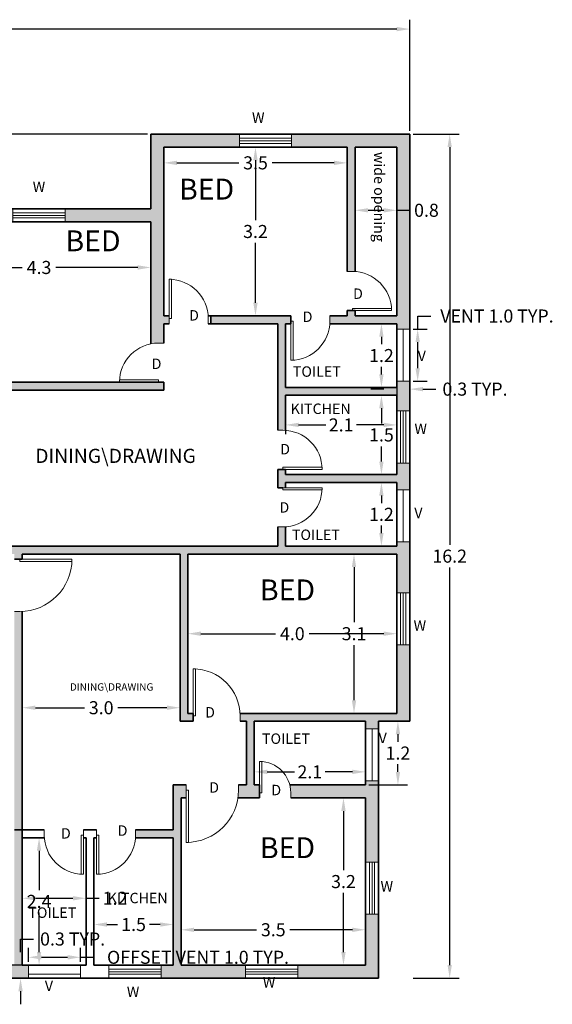
# Model space of a CAD drawing. Units: metres. Extents: x 6.2 to 29.4, y -2.1 to 16.8.
# Tile 3 of 3: x 19.2 to 29.4, y -2.1 to 16.8. Entities that reach past the tile are written whole.
import ezdxf

# ---------------------------------------------------------------- set-up
doc = ezdxf.new("R2010")
doc.units = ezdxf.units.M
doc.header["$MEASUREMENT"] = 0
doc.layers.get('0').update_dxf_attribs({"color": 2})
doc.layers.get('Defpoints').update_dxf_attribs({"color": 3})
for name, color, linetype, lineweight in [('A-ANNO-DIMS', 6, 'Continuous', 13), ('A-ANNO-TEXT', 7, 'Continuous', 18), ('A-AREA-IDEN', 3, 'Continuous', 18), ('A-DOOR', 3, 'Continuous', 18), ('A-GLAZ', 4, 'Continuous', 18), ('A-WALL', 7, 'Continuous', 35), ('A-WALL-PATT', 252, 'Continuous', 13)]:
    doc.layers.add(name, color=color, linetype=linetype, lineweight=lineweight)
doc.styles.get("Standard").update_dxf_attribs({"font": 'arial.ttf'})
doc.dimstyles.get("Standard").update_dxf_attribs({"dimtxt": 0.25, "dimasz": 0.25, "dimexe": 0.18, "dimexo": 0.0625, "dimgap": 0.09, "dimtad": 0, "dimtih": 1, "dimtoh": 1, "dimdec": 1, "dimzin": 0, "dimdsep": 46, "dimtxsty": 'Standard', "dimcen": 0.09, "dimadec": 0, "dimazin": 0, "dimtfac": 1, "dimtdec": 1, "dimtofl": 0, "dimtmove": 0, "dimatfit": 3, "dimfxl": 1, "dimtolj": 1, "dimtzin": 0, "dimarcsym": 0})

# ---------------------------------------------------------------- blocks, each defined once
blk = doc.blocks.new('*U11')
for p, q in [((-750, 0), (-750, 100)), ((0, 0), (0, 100))]:
    blk.add_line(p, q)
blk.add_lwpolyline([(0, 0), (0, -750), (-43.75, -750), (-43.75, 0)], close=True)
blk.add_arc((0, 0), 750, 180, 270)
blk = doc.blocks.new('*D12')
at = {"layer": 'A-ANNO-DIMS', "color": 0, "lineweight": -2, "transparency": 16777216}
for p, q in [((19.462, 1.113), (19.345, 1.113)), ((19.525, 0.863), (19.525, 0.109)), ((19.525, -1.077), (19.525, -0.322)), ((19.462, -1.327), (19.345, -1.327))]:
    blk.add_line(p, q, dxfattribs=at)
at = {"layer": 'A-ANNO-DIMS', "color": 0, "transparency": 16777216}
for points in [[(19.483, 0.863), (19.566, 0.863), (19.525, 1.113)], [(19.483, -1.077), (19.566, -1.077), (19.525, -1.327)]]:
    blk.add_solid(points, dxfattribs=at)
at = {"layer": 'Defpoints', "color": 0, "transparency": 16777216}
for p in [(19.525, 1.113), (19.525, -1.327), (19.525, -1.327)]:
    blk.add_point(p, dxfattribs=at)
at = {"layer": 'A-ANNO-DIMS', "color": 0, "transparency": 16777216, "insert": (19.525, -0.107), "char_height": 0.25, "attachment_point": 5}
blk.add_mtext('\\A1;2.4', dxfattribs=at)
blk = doc.blocks.new('*D13')
at = {"layer": 'A-ANNO-DIMS', "color": 0, "lineweight": -2, "transparency": 16777216}
for p, q in [((19.204, -0.087), (19.204, 0.133)), ((20.424, -1.149), (20.424, 0.133)), ((19.454, -0.047), (20.174, -0.047)), ((20.424, -0.047), (20.674, -0.047))]:
    blk.add_line(p, q, dxfattribs=at)
at = {"layer": 'A-ANNO-DIMS', "color": 0, "transparency": 16777216}
for points in [[(19.454, -0.005), (19.454, -0.088), (19.204, -0.047)], [(20.174, -0.005), (20.174, -0.088), (20.424, -0.047)]]:
    blk.add_solid(points, dxfattribs=at)
at = {"layer": 'Defpoints', "color": 0, "transparency": 16777216}
for p in [(19.204, -0.149), (20.424, -0.047), (20.424, -1.211)]:
    blk.add_point(p, dxfattribs=at)
at = {"layer": 'A-ANNO-DIMS', "color": 0, "transparency": 16777216, "insert": (20.979, -0.047), "char_height": 0.25, "attachment_point": 5}
blk.add_mtext('\\A1;1.2', dxfattribs=at)
blk = doc.blocks.new('*D14')
at = {"layer": 'A-ANNO-DIMS', "color": 0, "lineweight": -2, "transparency": 16777216}
for p, q in [((20.574, -0.487), (20.574, -0.369)), ((22.094, -0.487), (22.094, -0.369)), ((20.824, -0.549), (21.027, -0.549)), ((21.844, -0.549), (21.641, -0.549))]:
    blk.add_line(p, q, dxfattribs=at)
at = {"layer": 'A-ANNO-DIMS', "color": 0, "transparency": 16777216}
for points in [[(20.824, -0.508), (20.824, -0.591), (20.574, -0.549)], [(21.844, -0.508), (21.844, -0.591), (22.094, -0.549)]]:
    blk.add_solid(points, dxfattribs=at)
at = {"layer": 'Defpoints', "color": 0, "transparency": 16777216}
for p in [(20.574, -0.549), (22.094, -0.549), (22.094, -0.549)]:
    blk.add_point(p, dxfattribs=at)
at = {"layer": 'A-ANNO-DIMS', "color": 0, "transparency": 16777216, "insert": (21.334, -0.549), "char_height": 0.25, "attachment_point": 5}
blk.add_mtext('\\A1;1.5', dxfattribs=at)
blk = doc.blocks.new('*U15')
for p, q in [((0, 0), (0, 100)), ((1000, 0), (1000, 100))]:
    blk.add_line(p, q)
blk.add_lwpolyline([(0, 0), (0, -1000), (43.75, -1000), (43.75, 0)], close=True)
blk.add_arc((0, 0), 1000, 270, 0)
blk = doc.blocks.new('*D16')
at = {"layer": 'A-ANNO-DIMS', "color": 0, "lineweight": -2, "transparency": 16777216}
for p, q in [((22.244, -1.264), (22.244, -0.47)), ((25.774, -1.264), (25.774, -0.47)), ((22.494, -0.65), (23.691, -0.65)), ((25.524, -0.65), (24.328, -0.65))]:
    blk.add_line(p, q, dxfattribs=at)
at = {"layer": 'A-ANNO-DIMS', "color": 0, "transparency": 16777216}
for points in [[(22.494, -0.609), (22.494, -0.692), (22.244, -0.65)], [(25.524, -0.609), (25.524, -0.692), (25.774, -0.65)]]:
    blk.add_solid(points, dxfattribs=at)
at = {"layer": 'Defpoints', "color": 0, "transparency": 16777216}
for p in [(25.774, -0.65), (22.244, -1.327), (25.774, -1.327)]:
    blk.add_point(p, dxfattribs=at)
at = {"layer": 'A-ANNO-DIMS', "color": 0, "transparency": 16777216, "insert": (24.009, -0.65), "char_height": 0.25, "attachment_point": 5}
blk.add_mtext('\\A1;3.5', dxfattribs=at)
blk = doc.blocks.new('*U25')
for p, q in [((0, 0), (0, -100)), ((600, 0), (600, -100))]:
    blk.add_line(p, q)
blk.add_lwpolyline([(0, 0), (0, 600), (43.75, 600), (43.75, 0)], close=True)
blk.add_arc((0, 0), 600, 0, 90)
blk = doc.blocks.new('*D26')
at = {"layer": 'A-ANNO-DIMS', "color": 0, "lineweight": -2, "transparency": 16777216}
for p, q in [((26.562, 3.343), (26.216, 3.343)), ((26.396, 3.093), (26.396, 2.949)), ((26.396, 2.373), (26.396, 2.518)), ((25.837, 2.123), (26.576, 2.123))]:
    blk.add_line(p, q, dxfattribs=at)
at = {"layer": 'A-ANNO-DIMS', "color": 0, "transparency": 16777216}
for points in [[(26.354, 3.093), (26.438, 3.093), (26.396, 3.343)], [(26.354, 2.373), (26.438, 2.373), (26.396, 2.123)]]:
    blk.add_solid(points, dxfattribs=at)
at = {"layer": 'Defpoints', "color": 0, "transparency": 16777216}
for p in [(26.624, 3.343), (25.774, 2.123), (26.396, 2.123)]:
    blk.add_point(p, dxfattribs=at)
at = {"layer": 'A-ANNO-DIMS', "color": 0, "transparency": 16777216, "insert": (26.396, 2.733), "char_height": 0.25, "attachment_point": 5}
blk.add_mtext('\\A1;1.2', dxfattribs=at)
blk = doc.blocks.new('*D27')
at = {"layer": 'A-ANNO-DIMS', "color": 0, "lineweight": -2, "transparency": 16777216}
for p, q in [((23.644, 3.281), (23.644, 2.193)), ((25.774, 3.281), (25.774, 2.193)), ((23.894, 2.373), (24.414, 2.373)), ((25.524, 2.373), (25.005, 2.373))]:
    blk.add_line(p, q, dxfattribs=at)
at = {"layer": 'A-ANNO-DIMS', "color": 0, "transparency": 16777216}
for points in [[(23.894, 2.415), (23.894, 2.331), (23.644, 2.373)], [(25.524, 2.415), (25.524, 2.331), (25.774, 2.373)]]:
    blk.add_solid(points, dxfattribs=at)
at = {"layer": 'Defpoints', "color": 0, "transparency": 16777216}
for p in [(23.644, 3.343), (25.774, 3.343), (25.774, 2.373)]:
    blk.add_point(p, dxfattribs=at)
at = {"layer": 'A-ANNO-DIMS', "color": 0, "transparency": 16777216, "insert": (24.709, 2.373), "char_height": 0.25, "attachment_point": 5}
blk.add_mtext('\\A1;2.1', dxfattribs=at)
blk = doc.blocks.new('*D28')
at = {"layer": 'A-ANNO-DIMS', "color": 0, "lineweight": -2, "transparency": 16777216}
for p, q in [((25.712, 1.873), (25.173, 1.873)), ((25.353, 1.623), (25.353, 0.491)), ((25.353, -1.077), (25.353, 0.055)), ((25.712, -1.327), (25.173, -1.327))]:
    blk.add_line(p, q, dxfattribs=at)
at = {"layer": 'A-ANNO-DIMS', "color": 0, "transparency": 16777216}
for points in [[(25.311, 1.623), (25.395, 1.623), (25.353, 1.873)], [(25.311, -1.077), (25.395, -1.077), (25.353, -1.327)]]:
    blk.add_solid(points, dxfattribs=at)
at = {"layer": 'Defpoints', "color": 0, "transparency": 16777216}
for p in [(25.774, 1.873), (25.353, -1.327), (25.774, -1.327)]:
    blk.add_point(p, dxfattribs=at)
at = {"layer": 'A-ANNO-DIMS', "color": 0, "transparency": 16777216, "insert": (25.353, 0.273), "char_height": 0.25, "attachment_point": 5}
blk.add_mtext('\\A1;3.2', dxfattribs=at)
blk = doc.blocks.new('*U29')
for p, q in [((0, 0), (0, -100)), ((900, 0), (900, -100))]:
    blk.add_line(p, q)
blk.add_lwpolyline([(0, 0), (0, 900), (43.75, 900), (43.75, 0)], close=True)
blk.add_arc((0, 0), 900, 0, 90)
blk = doc.blocks.new('*D30')
at = {"layer": 'A-ANNO-DIMS', "color": 0, "lineweight": -2, "transparency": 16777216}
for p, q in [((22.374, 5.081), (22.374, 5.198)), ((26.374, 5.081), (26.374, 5.198)), ((22.624, 5.018), (24.052, 5.018)), ((26.124, 5.018), (24.696, 5.018))]:
    blk.add_line(p, q, dxfattribs=at)
at = {"layer": 'A-ANNO-DIMS', "color": 0, "transparency": 16777216}
for points in [[(22.624, 5.06), (22.624, 4.976), (22.374, 5.018)], [(26.124, 5.06), (26.124, 4.976), (26.374, 5.018)]]:
    blk.add_solid(points, dxfattribs=at)
at = {"layer": 'Defpoints', "color": 0, "transparency": 16777216}
for p in [(22.374, 5.018), (26.374, 5.018), (26.374, 5.018)]:
    blk.add_point(p, dxfattribs=at)
at = {"layer": 'A-ANNO-DIMS', "color": 0, "transparency": 16777216, "insert": (24.374, 5.018), "char_height": 0.25, "attachment_point": 5}
blk.add_mtext('\\A1;4.0', dxfattribs=at)
blk = doc.blocks.new('*D31')
at = {"layer": 'A-ANNO-DIMS', "color": 0, "lineweight": -2, "transparency": 16777216}
for p, q in [((25.905, 6.543), (25.375, 6.543)), ((25.555, 6.293), (25.555, 5.236)), ((25.555, 3.743), (25.555, 4.8)), ((25.905, 3.493), (25.375, 3.493))]:
    blk.add_line(p, q, dxfattribs=at)
at = {"layer": 'A-ANNO-DIMS', "color": 0, "transparency": 16777216}
for points in [[(25.513, 6.293), (25.597, 6.293), (25.555, 6.543)], [(25.513, 3.743), (25.597, 3.743), (25.555, 3.493)]]:
    blk.add_solid(points, dxfattribs=at)
at = {"layer": 'Defpoints', "color": 0, "transparency": 16777216}
for p in [(25.967, 6.543), (25.555, 3.493), (25.967, 3.493)]:
    blk.add_point(p, dxfattribs=at)
at = {"layer": 'A-ANNO-DIMS', "color": 0, "transparency": 16777216, "insert": (25.555, 5.018), "char_height": 0.25, "attachment_point": 5}
blk.add_mtext('\\A1;3.1', dxfattribs=at)
blk = doc.blocks.new('*D32')
at = {"layer": 'A-ANNO-DIMS', "color": 0, "lineweight": -2, "transparency": 16777216}
for p, q in [((19.204, 3.406), (19.204, 3.781)), ((22.224, 3.406), (22.224, 3.781)), ((19.454, 3.601), (20.397, 3.601)), ((21.974, 3.601), (21.031, 3.601))]:
    blk.add_line(p, q, dxfattribs=at)
at = {"layer": 'A-ANNO-DIMS', "color": 0, "transparency": 16777216}
for points in [[(19.454, 3.643), (19.454, 3.559), (19.204, 3.601)], [(21.974, 3.643), (21.974, 3.559), (22.224, 3.601)]]:
    blk.add_solid(points, dxfattribs=at)
at = {"layer": 'Defpoints', "color": 0, "transparency": 16777216}
for p in [(19.204, 3.601), (19.204, 3.343), (22.224, 3.343)]:
    blk.add_point(p, dxfattribs=at)
at = {"layer": 'A-ANNO-DIMS', "color": 0, "transparency": 16777216, "insert": (20.714, 3.601), "char_height": 0.25, "attachment_point": 5}
blk.add_mtext('\\A1;3.0', dxfattribs=at)
blk = doc.blocks.new('*U33')
for p, q in [((0, 0), (0, -100)), ((1000, 0), (1000, -100))]:
    blk.add_line(p, q)
blk.add_lwpolyline([(0, 0), (0, 1000), (43.75, 1000), (43.75, 0)], close=True)
blk.add_arc((0, 0), 1000, 0, 90)
blk = doc.blocks.new('*U36')
for p, q in [((-750, 0), (-750, -100)), ((0, 0), (0, -100))]:
    blk.add_line(p, q)
blk.add_lwpolyline([(0, 0), (0, 750), (-43.75, 750), (-43.75, 0)], close=True)
blk.add_arc((0, 0), 750, 90, 180)
blk = doc.blocks.new('*U34')
for p, q in [((0, 0), (0, -100)), ((750, 0), (750, -100))]:
    blk.add_line(p, q)
blk.add_lwpolyline([(0, 0), (0, 750), (43.75, 750), (43.75, 0)], close=True)
blk.add_arc((0, 0), 750, 0, 90)
blk = doc.blocks.new('*U35')
for p, q in [((-750, 0), (-750, -100)), ((0, 0), (0, -100))]:
    blk.add_line(p, q)
blk.add_lwpolyline([(0, 0), (0, 750), (-43.75, 750), (-43.75, 0)], close=True)
blk.add_arc((0, 0), 750, 90, 180)
blk = doc.blocks.new('*D37')
at = {"layer": 'A-ANNO-DIMS', "color": 0, "lineweight": -2, "transparency": 16777216}
for p, q in [((17.384, 12.84), (17.384, 11.849)), ((21.664, 12.84), (21.664, 11.849)), ((17.634, 12.029), (19.202, 12.029)), ((21.414, 12.029), (19.847, 12.029))]:
    blk.add_line(p, q, dxfattribs=at)
at = {"layer": 'A-ANNO-DIMS', "color": 0, "transparency": 16777216}
for points in [[(17.634, 12.071), (17.634, 11.987), (17.384, 12.029)], [(21.414, 12.071), (21.414, 11.987), (21.664, 12.029)]]:
    blk.add_solid(points, dxfattribs=at)
at = {"layer": 'Defpoints', "color": 0, "transparency": 16777216}
for p in [(17.384, 12.903), (21.664, 12.903), (21.664, 12.029)]:
    blk.add_point(p, dxfattribs=at)
at = {"layer": 'A-ANNO-DIMS', "color": 0, "transparency": 16777216, "insert": (19.524, 12.029), "char_height": 0.25, "attachment_point": 5}
blk.add_mtext('\\A1;4.3', dxfattribs=at)
blk = doc.blocks.new('*D38')
at = {"layer": 'A-ANNO-DIMS', "color": 0, "lineweight": -2, "transparency": 16777216}
for p, q in [((21.914, 14.271), (21.914, 13.852)), ((25.424, 14.271), (25.424, 13.852)), ((22.164, 14.032), (23.351, 14.032)), ((25.174, 14.032), (23.988, 14.032))]:
    blk.add_line(p, q, dxfattribs=at)
at = {"layer": 'A-ANNO-DIMS', "color": 0, "transparency": 16777216}
for points in [[(22.164, 14.073), (22.164, 13.99), (21.914, 14.032)], [(25.174, 14.073), (25.174, 13.99), (25.424, 14.032)]]:
    blk.add_solid(points, dxfattribs=at)
at = {"layer": 'Defpoints', "color": 0, "transparency": 16777216}
for p in [(21.914, 14.333), (25.424, 14.333), (25.424, 14.032)]:
    blk.add_point(p, dxfattribs=at)
at = {"layer": 'A-ANNO-DIMS', "color": 0, "transparency": 16777216, "insert": (23.669, 14.032), "char_height": 0.25, "attachment_point": 5}
blk.add_mtext('\\A1;3.5', dxfattribs=at)
blk = doc.blocks.new('*D39')
at = {"layer": 'A-ANNO-DIMS', "color": 0, "lineweight": -2, "transparency": 16777216}
for p, q in [((23.607, 14.333), (23.488, 14.333)), ((23.668, 14.083), (23.668, 12.936)), ((23.668, 11.353), (23.668, 12.5)), ((23.616, 11.103), (23.848, 11.103))]:
    blk.add_line(p, q, dxfattribs=at)
at = {"layer": 'A-ANNO-DIMS', "color": 0, "transparency": 16777216}
for points in [[(23.627, 14.083), (23.71, 14.083), (23.668, 14.333)], [(23.627, 11.353), (23.71, 11.353), (23.668, 11.103)]]:
    blk.add_solid(points, dxfattribs=at)
at = {"layer": 'Defpoints', "color": 0, "transparency": 16777216}
for p in [(23.668, 14.333), (23.669, 14.333), (23.553, 11.103)]:
    blk.add_point(p, dxfattribs=at)
at = {"layer": 'A-ANNO-DIMS', "color": 0, "transparency": 16777216, "insert": (23.668, 12.718), "char_height": 0.25, "attachment_point": 5}
blk.add_mtext('\\A1;3.2', dxfattribs=at)
blk = doc.blocks.new('*D40')
at = {"layer": 'A-ANNO-DIMS', "color": 0, "lineweight": -2, "transparency": 16777216}
for p, q in [((25.574, 12.748), (25.574, 13.304)), ((26.374, 12.748), (26.374, 13.304)), ((25.824, 13.124), (26.124, 13.124)), ((26.374, 13.124), (26.624, 13.124))]:
    blk.add_line(p, q, dxfattribs=at)
at = {"layer": 'A-ANNO-DIMS', "color": 0, "transparency": 16777216}
for points in [[(25.824, 13.165), (25.824, 13.082), (25.574, 13.124)], [(26.124, 13.165), (26.124, 13.082), (26.374, 13.124)]]:
    blk.add_solid(points, dxfattribs=at)
at = {"layer": 'Defpoints', "color": 0, "transparency": 16777216}
for p in [(26.374, 13.124), (25.574, 12.686), (26.374, 12.686)]:
    blk.add_point(p, dxfattribs=at)
at = {"layer": 'A-ANNO-DIMS', "color": 0, "transparency": 16777216, "insert": (26.942, 13.124), "char_height": 0.25, "attachment_point": 5}
blk.add_mtext('\\A1;0.8', dxfattribs=at)
blk = doc.blocks.new('*D41')
at = {"layer": 'A-ANNO-DIMS', "color": 0, "lineweight": -2, "transparency": 16777216}
for p, q in [((26.312, 10.953), (25.9, 10.953)), ((26.08, 10.703), (26.08, 10.559)), ((26.08, 9.983), (26.08, 10.128)), ((26.312, 9.733), (25.9, 9.733))]:
    blk.add_line(p, q, dxfattribs=at)
at = {"layer": 'A-ANNO-DIMS', "color": 0, "transparency": 16777216}
for points in [[(26.038, 10.703), (26.121, 10.703), (26.08, 10.953)], [(26.038, 9.983), (26.121, 9.983), (26.08, 9.733)]]:
    blk.add_solid(points, dxfattribs=at)
at = {"layer": 'Defpoints', "color": 0, "transparency": 16777216}
for p in [(26.374, 10.953), (26.08, 9.733), (26.374, 9.733)]:
    blk.add_point(p, dxfattribs=at)
at = {"layer": 'A-ANNO-DIMS', "color": 0, "transparency": 16777216, "insert": (26.08, 10.343), "char_height": 0.25, "attachment_point": 5}
blk.add_mtext('\\A1;1.2', dxfattribs=at)
blk = doc.blocks.new('*D42')
at = {"layer": 'A-ANNO-DIMS', "color": 0, "lineweight": -2, "transparency": 16777216}
for p, q in [((26.017, 9.583), (25.9, 9.583)), ((26.08, 9.333), (26.08, 9.041)), ((26.08, 8.313), (26.08, 8.605)), ((26.017, 8.063), (25.9, 8.063))]:
    blk.add_line(p, q, dxfattribs=at)
at = {"layer": 'A-ANNO-DIMS', "color": 0, "transparency": 16777216}
for points in [[(26.038, 9.333), (26.121, 9.333), (26.08, 9.583)], [(26.038, 8.313), (26.121, 8.313), (26.08, 8.063)]]:
    blk.add_solid(points, dxfattribs=at)
at = {"layer": 'Defpoints', "color": 0, "transparency": 16777216}
for p in [(26.08, 9.583), (26.08, 8.063), (26.08, 8.063)]:
    blk.add_point(p, dxfattribs=at)
at = {"layer": 'A-ANNO-DIMS', "color": 0, "transparency": 16777216, "insert": (26.08, 8.823), "char_height": 0.25, "attachment_point": 5}
blk.add_mtext('\\A1;1.5', dxfattribs=at)
blk = doc.blocks.new('*D43')
at = {"layer": 'A-ANNO-DIMS', "color": 0, "lineweight": -2, "transparency": 16777216}
for p, q in [((26.017, 7.913), (25.9, 7.913)), ((26.08, 7.663), (26.08, 7.519)), ((26.08, 6.943), (26.08, 7.088)), ((26.017, 6.693), (25.9, 6.693))]:
    blk.add_line(p, q, dxfattribs=at)
at = {"layer": 'A-ANNO-DIMS', "color": 0, "transparency": 16777216}
for points in [[(26.038, 7.663), (26.121, 7.663), (26.08, 7.913)], [(26.038, 6.943), (26.121, 6.943), (26.08, 6.693)]]:
    blk.add_solid(points, dxfattribs=at)
at = {"layer": 'Defpoints', "color": 0, "transparency": 16777216}
for p in [(26.08, 7.913), (26.08, 6.693), (26.08, 6.693)]:
    blk.add_point(p, dxfattribs=at)
at = {"layer": 'A-ANNO-DIMS', "color": 0, "transparency": 16777216, "insert": (26.08, 7.303), "char_height": 0.25, "attachment_point": 5}
blk.add_mtext('\\A1;1.2', dxfattribs=at)
blk = doc.blocks.new('*D44')
at = {"layer": 'A-ANNO-DIMS', "color": 0, "lineweight": -2, "transparency": 16777216}
for p, q in [((24.244, 9.185), (24.244, 8.835)), ((26.374, 9.185), (26.374, 8.835)), ((24.494, 9.015), (25.014, 9.015)), ((26.124, 9.015), (25.605, 9.015))]:
    blk.add_line(p, q, dxfattribs=at)
at = {"layer": 'A-ANNO-DIMS', "color": 0, "transparency": 16777216}
for points in [[(24.494, 9.057), (24.494, 8.974), (24.244, 9.015)], [(26.124, 9.057), (26.124, 8.974), (26.374, 9.015)]]:
    blk.add_solid(points, dxfattribs=at)
at = {"layer": 'Defpoints', "color": 0, "transparency": 16777216}
for p in [(24.244, 9.247), (26.374, 9.247), (26.374, 9.015)]:
    blk.add_point(p, dxfattribs=at)
at = {"layer": 'A-ANNO-DIMS', "color": 0, "transparency": 16777216, "insert": (25.309, 9.015), "char_height": 0.25, "attachment_point": 5}
blk.add_mtext('\\A1;2.1', dxfattribs=at)
blk = doc.blocks.new('*D59')
at = {"layer": 'A-ANNO-DIMS', "color": 0, "lineweight": -2, "transparency": 16777216}
for p, q in [((7.674, 11.556), (7.674, 16.773)), ((7.924, 16.593), (16.746, 16.593)), ((26.374, 16.593), (17.551, 16.593)), ((26.624, 14.646), (26.624, 16.773))]:
    blk.add_line(p, q, dxfattribs=at)
at = {"layer": 'A-ANNO-DIMS', "color": 0, "transparency": 16777216}
for points in [[(7.924, 16.634), (7.924, 16.551), (7.674, 16.593)], [(26.374, 16.634), (26.374, 16.551), (26.624, 16.593)]]:
    blk.add_solid(points, dxfattribs=at)
at = {"layer": 'Defpoints', "color": 0, "transparency": 16777216}
for p in [(7.674, 16.593), (26.624, 14.583), (7.674, 11.494)]:
    blk.add_point(p, dxfattribs=at)
at = {"layer": 'A-ANNO-DIMS', "color": 0, "transparency": 16777216, "insert": (17.149, 16.593), "char_height": 0.25, "attachment_point": 5}
blk.add_mtext('\\A1;19.0', dxfattribs=at)
blk = doc.blocks.new('*D61')
at = {"layer": 'A-ANNO-DIMS', "color": 0, "lineweight": -2, "transparency": 16777216}
for p, q in [((26.687, 14.583), (27.567, 14.583)), ((27.387, 14.333), (27.387, 6.721)), ((27.387, -1.327), (27.387, 6.285)), ((26.687, -1.577), (27.567, -1.577))]:
    blk.add_line(p, q, dxfattribs=at)
at = {"layer": 'A-ANNO-DIMS', "color": 0, "transparency": 16777216}
for points in [[(27.345, 14.333), (27.428, 14.333), (27.387, 14.583)], [(27.345, -1.327), (27.428, -1.327), (27.387, -1.577)]]:
    blk.add_solid(points, dxfattribs=at)
at = {"layer": 'Defpoints', "color": 0, "transparency": 16777216}
for p in [(26.624, 14.583), (26.624, -1.577), (27.387, -1.577)]:
    blk.add_point(p, dxfattribs=at)
at = {"layer": 'A-ANNO-DIMS', "color": 0, "transparency": 16777216, "insert": (27.387, 6.503), "char_height": 0.25, "attachment_point": 5}
blk.add_mtext('\\A1;16.2', dxfattribs=at)
blk = doc.blocks.new('WIN-1000')
for p, q in [((0.075, 1), (0.075, 0)), ((0.125, 1), (0.125, 0)), ((0.175, 1), (0.175, 0))]:
    blk.add_line(p, q)
blk.add_lwpolyline([(0, 1), (0.25, 1), (0.25, 0), (0, 0)], close=True)
blk = doc.blocks.new('VENT-1000')
blk.add_line((0.125, 1), (0.125, 0))
blk.add_lwpolyline([(0, 1), (0.25, 1), (0.25, 0), (0, 0)], close=True)
blk = doc.blocks.new('VENT-1000-OFFSET')
blk.add_line((0, 0.075), (1, 0.075))
blk.add_lwpolyline([(0, 0.25), (1, 0.25), (1, 0), (0, 0)], close=True)
blk = doc.blocks.new('*D67')
at = {"layer": 'A-ANNO-DIMS', "color": 0, "lineweight": -2, "transparency": 16777216}
for p, q in [((26.774, 10.85), (26.774, 11.1)), ((26.774, 11.1), (27.024, 11.1)), ((26.686, 10.85), (26.954, 10.85)), ((26.774, 10.1), (26.774, 10.6)), ((26.686, 9.85), (26.954, 9.85))]:
    blk.add_line(p, q, dxfattribs=at)
at = {"layer": 'A-ANNO-DIMS', "color": 0, "transparency": 16777216}
for points in [[(26.732, 10.6), (26.816, 10.6), (26.774, 10.85)], [(26.732, 10.1), (26.816, 10.1), (26.774, 9.85)]]:
    blk.add_solid(points, dxfattribs=at)
at = {"layer": 'Defpoints', "color": 0, "transparency": 16777216}
for p in [(26.624, 10.85), (26.774, 10.85), (26.624, 9.85)]:
    blk.add_point(p, dxfattribs=at)
at = {"layer": 'A-ANNO-DIMS', "color": 0, "transparency": 16777216, "insert": (28.292, 11.1), "char_height": 0.25, "attachment_point": 5}
blk.add_mtext('\\A1;VENT 1.0 TYP.', dxfattribs=at)
blk = doc.blocks.new('*D68')
at = {"layer": 'A-ANNO-DIMS', "color": 0, "lineweight": -2, "transparency": 16777216}
for p, q in [((26.124, 9.7), (25.874, 9.7)), ((26.374, 9.787), (26.374, 9.52)), ((26.624, 9.787), (26.624, 9.52)), ((26.874, 9.7), (27.124, 9.7))]:
    blk.add_line(p, q, dxfattribs=at)
at = {"layer": 'A-ANNO-DIMS', "color": 0, "transparency": 16777216}
for points in [[(26.124, 9.741), (26.124, 9.658), (26.374, 9.7)], [(26.874, 9.741), (26.874, 9.658), (26.624, 9.7)]]:
    blk.add_solid(points, dxfattribs=at)
at = {"layer": 'Defpoints', "color": 0, "transparency": 16777216}
for p in [(26.374, 9.85), (26.624, 9.85), (26.624, 9.7)]:
    blk.add_point(p, dxfattribs=at)
at = {"layer": 'A-ANNO-DIMS', "color": 0, "transparency": 16777216, "insert": (27.871, 9.7), "char_height": 0.25, "attachment_point": 5}
blk.add_mtext('\\A1;0.3 TYP.', dxfattribs=at)
blk = doc.blocks.new('*D69')
at = {"layer": 'A-ANNO-DIMS', "color": 0, "lineweight": -2, "transparency": 16777216}
for p, q in [((19.32, -1.264), (19.32, -0.997)), ((20.32, -1.264), (20.32, -0.997)), ((19.57, -1.177), (20.07, -1.177)), ((20.32, -1.177), (20.57, -1.177))]:
    blk.add_line(p, q, dxfattribs=at)
at = {"layer": 'A-ANNO-DIMS', "color": 0, "transparency": 16777216}
for points in [[(19.57, -1.135), (19.57, -1.219), (19.32, -1.177)], [(20.07, -1.135), (20.07, -1.219), (20.32, -1.177)]]:
    blk.add_solid(points, dxfattribs=at)
at = {"layer": 'Defpoints', "color": 0, "transparency": 16777216}
for p in [(20.32, -1.177), (19.32, -1.327), (20.32, -1.327)]:
    blk.add_point(p, dxfattribs=at)
at = {"layer": 'A-ANNO-DIMS', "color": 0, "transparency": 16777216, "insert": (22.568, -1.177), "char_height": 0.25, "attachment_point": 5}
blk.add_mtext('\\A1;OFFSET VENT 1.0 TYP.', dxfattribs=at)
blk = doc.blocks.new('*D70')
at = {"layer": 'A-ANNO-DIMS', "color": 0, "lineweight": -2, "transparency": 16777216}
for p, q in [((19.17, -1.077), (19.17, -0.827)), ((19.17, -0.827), (19.42, -0.827)), ((19.258, -1.327), (18.99, -1.327)), ((19.258, -1.577), (18.99, -1.577)), ((19.17, -1.827), (19.17, -2.077))]:
    blk.add_line(p, q, dxfattribs=at)
at = {"layer": 'A-ANNO-DIMS', "color": 0, "transparency": 16777216}
for points in [[(19.129, -1.077), (19.212, -1.077), (19.17, -1.327)], [(19.129, -1.827), (19.212, -1.827), (19.17, -1.577)]]:
    blk.add_solid(points, dxfattribs=at)
at = {"layer": 'Defpoints', "color": 0, "transparency": 16777216}
for p in [(19.17, -1.327), (19.32, -1.327), (19.32, -1.577)]:
    blk.add_point(p, dxfattribs=at)
at = {"layer": 'A-ANNO-DIMS', "color": 0, "transparency": 16777216, "insert": (20.167, -0.827), "char_height": 0.25, "attachment_point": 5}
blk.add_mtext('\\A1;0.3 TYP.', dxfattribs=at)
blk = doc.blocks.new('*D72')
at = {"layer": 'A-ANNO-DIMS', "color": 0, "lineweight": -2, "transparency": 16777216}
for p, q in [((21.602, 14.583), (6.408, 14.583)), ((6.588, 14.333), (6.588, 14.086)), ((6.588, 13.403), (6.588, 13.65)), ((21.602, 13.153), (6.408, 13.153))]:
    blk.add_line(p, q, dxfattribs=at)
at = {"layer": 'A-ANNO-DIMS', "color": 0, "transparency": 16777216}
for points in [[(6.546, 14.333), (6.63, 14.333), (6.588, 14.583)], [(6.546, 13.403), (6.63, 13.403), (6.588, 13.153)]]:
    blk.add_solid(points, dxfattribs=at)
at = {"layer": 'Defpoints', "color": 0, "transparency": 16777216}
for p in [(6.588, 14.583), (21.664, 14.583), (21.664, 13.153)]:
    blk.add_point(p, dxfattribs=at)
at = {"layer": 'A-ANNO-DIMS', "color": 0, "transparency": 16777216, "insert": (6.588, 13.868), "char_height": 0.25, "attachment_point": 5}
blk.add_mtext('\\A1;1.43', dxfattribs=at)

msp = doc.modelspace()

# ---------------------------------------------------------------- hatches: boundary and pattern name
at = {"layer": 'A-WALL-PATT'}
h = msp.add_hatch(dxfattribs=at)
h.set_pattern_fill('BRICK', color=256, scale=0.3)
h.paths.add_polyline_path([(26.024, -0.354), (25.774, -0.354), (25.774, -1.327), (24.478, -1.327), (24.478, -1.577), (26.024, -1.577)])
h.paths.add_polyline_path([(26.024, 2.199), (25.774, 2.199), (25.774, 2.123), (24.325, 2.123, -0.063254), (24.344, 1.973), (24.344, 1.873), (25.774, 1.873), (25.774, 0.646), (26.024, 0.646)])
h.paths.add_polyline_path([(26.624, 4.802), (26.374, 4.802), (26.374, 3.493), (23.373, 3.493, -0.013897), (23.374, 3.443), (23.374, 3.343), (23.494, 3.343), (23.494, 2.123), (23.344, 2.123), (23.344, 2.023, -0.03766), (23.333, 1.873), (23.744, 1.873), (23.744, 1.973), (23.744, 2.123), (23.644, 2.123), (23.644, 3.343), (25.774, 3.343), (25.774, 3.199), (26.024, 3.199), (26.024, 3.343), (26.624, 3.343)])
h.paths.add_polyline_path([(26.624, 6.775), (26.374, 6.775), (26.374, 6.693), (24.244, 6.693), (24.244, 7.065, -0.016681), (24.194, 7.063), (24.094, 7.063), (24.094, 6.693), (19.054, 6.693), (19.054, 6.443), (19.154, 6.443), (19.204, 6.443), (19.204, 6.543), (22.224, 6.543), (22.224, 3.343), (22.474, 3.343), (22.474, 3.443), (22.474, 3.493), (22.374, 3.493), (22.374, 6.543), (26.374, 6.543), (26.374, 5.802), (26.624, 5.802)])
h.paths.add_polyline_path([(26.624, 8.282), (26.374, 8.282), (26.374, 8.063), (24.244, 8.063), (24.244, 8.163), (24.194, 8.163), (24.094, 8.163), (24.094, 7.813), (24.194, 7.813), (24.244, 7.813), (24.244, 7.913), (26.374, 7.913), (26.374, 7.775), (26.624, 7.775)])
h.paths.add_polyline_path([(26.624, 9.85), (26.374, 9.85), (26.374, 9.733), (24.244, 9.733), (24.244, 10.953), (24.344, 10.953), (24.344, 11.003), (24.344, 11.103), (22.814, 11.103), (22.814, 10.953), (24.094, 10.953), (24.094, 8.913), (24.194, 8.913, -0.016681), (24.244, 8.911), (24.244, 9.583), (26.374, 9.583), (26.374, 9.282), (26.624, 9.282)])
h.paths.add_polyline_path([(26.624, 14.583), (24.36, 14.583), (24.36, 14.333), (25.424, 14.333), (25.424, 11.953), (25.524, 11.953, -0.016681), (25.574, 11.951), (25.574, 14.333), (26.374, 14.333), (26.374, 11.103), (25.574, 11.103), (25.574, 11.203), (25.524, 11.203), (25.424, 11.203), (25.424, 11.103), (25.094, 11.103), (25.094, 11.003, -0.016681), (25.092, 10.953), (26.374, 10.953), (26.374, 10.85), (26.624, 10.85)])
h.paths.add_polyline_path([(23.36, 14.583), (21.664, 14.583), (21.664, 13.153), (20.023, 13.153), (20.023, 12.903), (21.664, 12.903), (21.664, 10.568, -0.050382), (21.814, 10.583), (21.914, 10.583), (21.914, 10.953), (22.014, 10.953), (22.014, 11.053), (22.014, 11.103), (21.914, 11.103), (21.914, 14.333), (23.36, 14.333)])
h.paths.add_polyline_path([(19.023, 13.153), (17.234, 13.153), (17.234, 12.453), (15.201, 12.453), (15.201, 12.203), (17.234, 12.203), (17.234, 8.643), (17.234, 6.543), (17.484, 6.543), (17.484, 6.643), (17.484, 6.693), (17.384, 6.693), (17.384, 9.683), (21.914, 9.683), (21.914, 9.833), (21.814, 9.833), (21.064, 9.833), (17.384, 9.833), (17.384, 12.903), (19.023, 12.903)])
h.paths.add_polyline_path([(14.201, 12.453), (12.964, 12.453), (12.964, 11.878), (12.801, 11.878), (12.801, 11.628), (12.964, 11.628), (12.964, 9.628), (11.744, 9.628), (11.744, 9.728), (11.694, 9.728), (11.594, 9.728), (11.594, 9.236, -0.016681), (11.644, 9.238), (11.744, 9.238), (11.744, 9.478), (12.964, 9.478), (12.964, 8.493), (13.214, 8.493), (13.214, 8.593), (13.214, 8.643), (13.114, 8.643), (13.114, 12.203), (14.201, 12.203)])
h.paths.add_polyline_path([(11.801, 11.878), (11.594, 11.878), (11.594, 11.494), (8.294, 11.494), (8.294, 10.872), (8.394, 10.872), (8.394, 11.378), (11.594, 11.378), (11.594, 10.478), (11.694, 10.478, -0.016681), (11.744, 10.476), (11.744, 11.628), (11.801, 11.628)])
h.paths.add_polyline_path([(8.394, 9.872), (8.294, 9.872), (8.294, 9.088), (8.394, 9.088)])
h.paths.add_polyline_path([(7.984, 7.122), (7.734, 7.122), (7.734, 6.491), (7.984, 6.491), (7.984, 6.658), (9.964, 6.658), (10.014, 6.658), (10.114, 6.658), (10.114, 6.808), (10.014, 6.808), (9.414, 6.808), (7.984, 6.808)])
h.paths.add_polyline_path([(7.984, 5.491), (7.734, 5.491), (7.734, 4.503), (7.984, 4.503), (7.984, 4.713), (9.964, 4.713), (9.964, 4.041, -0.016681), (10.014, 4.043), (10.114, 4.043), (10.114, 4.713), (16.404, 4.713), (16.404, 4.613), (16.454, 4.613), (16.554, 4.613), (16.554, 4.863), (10.114, 4.863), (10.114, 6.058), (10.014, 6.058, -0.020861), (9.964, 6.06), (9.964, 4.863), (7.984, 4.863)])
h.paths.add_polyline_path([(10.114, 3.293), (10.014, 3.293), (9.964, 3.293), (9.964, 3.193), (7.984, 3.193), (7.984, 3.503), (7.734, 3.503), (7.734, 2.884), (7.984, 2.884), (7.984, 3.043), (9.964, 3.043), (9.964, 2.943), (10.014, 2.943), (10.114, 2.943)])
h.paths.add_polyline_path([(7.984, 1.673), (10.216, 1.673, -0.013897), (10.214, 1.723), (10.214, 1.823), (10.114, 1.823), (10.114, 2.193), (10.014, 2.193, -0.016681), (9.964, 2.195), (9.964, 1.823), (7.984, 1.823), (7.984, 1.884), (7.734, 1.884), (7.734, 0.646), (7.984, 0.646)])
h.paths.add_polyline_path([(8.755, -1.327), (7.984, -1.327), (7.984, -0.354), (7.734, -0.354), (7.734, -1.577), (8.755, -1.577)])
h.paths.add_polyline_path([(11.615, -1.327), (11.364, -1.327), (11.364, -0.065, -0.020861), (11.314, -0.067), (11.214, -0.067), (11.214, -1.327), (9.755, -1.327), (9.755, -1.577), (11.615, -1.577)])
h.paths.add_polyline_path([(14.209, -1.327), (12.734, -1.327), (12.734, 0.875, -0.015636), (12.684, 0.873), (12.584, 0.873), (12.584, 0.783), (11.364, 0.783), (11.364, 1.823), (11.114, 1.823), (11.114, 1.723), (11.114, 1.673), (11.214, 1.673), (11.214, 0.533), (11.314, 0.533), (11.364, 0.533), (11.364, 0.633), (12.584, 0.633), (12.584, -1.327), (12.227, -1.327), (12.227, -1.577), (14.209, -1.577)])
h.paths.add_polyline_path([(17.304, -1.327), (16.554, -1.327), (16.554, 3.613), (16.454, 3.613, -0.012506), (16.404, 3.614), (16.404, 1.823), (12.584, 1.823), (12.584, 1.673), (12.684, 1.673), (13.484, 1.673), (16.404, 1.673), (16.404, -1.327), (15.209, -1.327), (15.209, -1.577), (17.304, -1.577)])
h.paths.add_polyline_path([(19.32, -1.327), (19.204, -1.327), (19.204, 1.263), (19.054, 1.263), (19.054, -1.327), (18.304, -1.327), (18.304, -1.577), (19.32, -1.577)])
h.paths.add_polyline_path([(23.478, -1.327), (22.244, -1.327), (22.244, 1.873), (22.344, 1.873), (22.344, 2.023), (22.344, 2.123), (22.094, 2.123), (22.094, 1.263), (21.374, 1.263), (21.374, 1.163, -0.016681), (21.372, 1.113), (22.094, 1.113), (22.094, -1.327), (21.86, -1.327), (21.86, -1.577), (23.478, -1.577)])
h.paths.add_polyline_path([(19.204, 5.444, -0.012506), (19.154, 5.443), (19.054, 5.443), (19.054, 1.263), (19.204, 1.263)])
h.paths.add_polyline_path([(19.054, 6.693), (18.483, 6.693, -0.012506), (18.484, 6.643), (18.484, 6.543), (19.054, 6.543)], flags=17)
h.paths.add_polyline_path([(11.744, 8.488), (7.674, 8.488), (7.674, 8.338), (7.734, 8.338), (7.734, 8.122), (7.984, 8.122), (7.984, 8.338), (9.964, 8.338), (9.964, 7.406, -0.020861), (10.014, 7.408), (10.114, 7.408), (10.114, 8.338), (11.744, 8.338)])
h.paths.add_polyline_path([(15.131, 11.42), (16.48, 11.42), (16.48, 12.245), (15.131, 12.245)], flags=9)
h.paths.add_polyline_path([(8.62, 7.608), (9.947, 7.608), (9.947, 8.021), (8.62, 8.021)], flags=24)

# ---------------------------------------------------------------- linework, layer by layer
at = {"layer": 'A-DOOR'}
for p, q in [((22.344, 1.273), (22.344, 1.873)), ((20.374, 0.413), (20.374, 1.263)), ((20.624, 0.413), (20.624, 1.263))]:
    msp.add_line(p, q, dxfattribs=at)
at = {"layer": 'A-WALL'}
for p, q in [((26.624, 14.583), (21.664, 14.583)), ((21.664, 14.583), (21.664, 13.153)), ((26.624, 14.583), (26.624, 3.343)), ((21.914, 14.333), (21.914, 11.103)), ((25.424, 14.333), (21.914, 14.333)), ((25.424, 14.333), (25.424, 11.953)), ((25.574, 14.333), (25.574, 11.951)), ((26.374, 14.333), (25.574, 14.333)), ((26.374, 14.333), (26.374, 11.103)), ((17.234, 13.153), (21.664, 13.153)), ((17.384, 12.903), (21.664, 12.903)), ((21.664, 12.903), (21.664, 10.568)), ((25.424, 11.203), (25.574, 11.203)), ((25.424, 11.203), (25.424, 11.103)), ((25.574, 11.203), (25.574, 11.103)), ((22.014, 11.103), (21.914, 11.103)), ((22.014, 10.953), (21.914, 10.953)), ((21.914, 10.953), (21.914, 10.583)), ((24.344, 11.103), (22.762, 11.103)), ((24.094, 10.953), (22.764, 10.953)), ((22.814, 11.103), (22.814, 10.953)), ((24.094, 10.953), (24.094, 8.913)), ((24.244, 10.953), (24.244, 9.733)), ((24.344, 10.953), (24.244, 10.953)), ((24.344, 10.953), (24.244, 10.953)), ((24.344, 10.953), (24.344, 11.103)), ((26.374, 10.953), (25.092, 10.953)), ((25.424, 11.103), (25.094, 11.103)), ((26.374, 11.103), (25.574, 11.103)), ((26.374, 10.953), (26.374, 9.733)), ((17.384, 9.833), (21.914, 9.833)), ((21.914, 9.833), (21.914, 9.683)), ((17.384, 9.683), (21.914, 9.683)), ((26.374, 9.733), (24.244, 9.733)), ((26.374, 9.583), (24.244, 9.583)), ((24.244, 9.583), (24.244, 8.911)), ((26.374, 9.583), (26.374, 8.063)), ((24.244, 8.163), (24.094, 8.163)), ((24.094, 8.163), (24.094, 7.813)), ((24.244, 8.163), (24.244, 8.063)), ((26.374, 8.063), (24.244, 8.063)), ((24.194, 7.813), (24.094, 7.813)), ((26.374, 7.913), (24.244, 7.913)), ((24.244, 7.913), (24.244, 7.813)), ((26.374, 7.913), (26.374, 6.693)), ((24.094, 7.063), (24.094, 6.693)), ((24.244, 7.065), (24.244, 6.693)), ((24.094, 6.693), (18.483, 6.693)), ((26.374, 6.693), (24.244, 6.693)), ((19.204, 6.443), (19.054, 6.443)), ((22.224, 6.543), (19.204, 6.543)), ((19.204, 6.443), (19.204, 6.543)), ((22.224, 6.543), (22.224, 3.343)), ((26.374, 6.543), (22.374, 6.543)), ((22.374, 6.543), (22.374, 3.493)), ((26.374, 6.543), (26.374, 3.493)), ((19.204, -1.327), (19.204, 5.444)), ((22.474, 3.493), (22.374, 3.493)), ((22.474, 3.493), (22.474, 3.343)), ((26.374, 3.493), (23.373, 3.493)), ((22.474, 3.343), (22.224, 3.343)), ((23.494, 3.343), (23.374, 3.343)), ((23.494, 2.123), (23.494, 3.343)), ((23.644, 2.123), (23.644, 3.343)), ((25.774, 3.343), (23.644, 3.343)), ((25.774, 2.123), (25.774, 3.343)), ((26.024, -1.577), (26.024, 3.343)), ((26.624, 3.343), (26.024, 3.343)), ((22.094, 1.263), (22.094, 2.123)), ((22.344, 2.123), (22.094, 2.123)), ((23.494, 2.123), (23.344, 2.123)), ((23.744, 2.123), (23.644, 2.123)), ((23.744, 2.123), (23.744, 1.873)), ((25.774, 2.123), (24.325, 2.123)), ((22.244, -1.327), (22.244, 1.873)), ((22.344, 1.873), (22.244, 1.873)), ((23.744, 1.873), (23.333, 1.873)), ((25.774, 1.873), (24.344, 1.873)), ((25.774, -1.327), (25.774, 1.873)), ((19.624, 1.263), (19.054, 1.263)), ((20.624, 1.263), (20.374, 1.263)), ((22.094, 1.263), (21.374, 1.263)), ((19.626, 1.113), (19.204, 1.113)), ((20.424, 1.113), (20.374, 1.113)), ((20.424, -1.327), (20.424, 1.113)), ((20.574, -1.327), (20.574, 1.113)), ((20.624, 1.113), (20.574, 1.113)), ((22.094, 1.113), (21.372, 1.113)), ((22.094, -1.327), (22.094, 1.113)), ((20.424, -1.327), (19.204, -1.327)), ((22.094, -1.327), (20.574, -1.327)), ((25.774, -1.327), (22.244, -1.327)), ((26.024, -1.577), (7.734, -1.577))]:
    msp.add_line(p, q, dxfattribs=at)

# ---------------------------------------------------------------- block references
at = {"layer": 'A-DOOR', "xscale": 0.001, "yscale": 0.001, "zscale": 0.001}
for name, p, rotation in [('*U36', (25.524, 11.203), 270), ('*U35', (24.344, 11.003), 180), ('*U34', (21.814, 9.833), 90), ('*U36', (24.194, 8.163), 270), ('*U34', (24.194, 7.813), 270), ('*U33', (19.154, 6.443), 270)]:
    msp.add_blockref(name, p, dxfattribs=dict(at, rotation=rotation))
at = {"layer": 'A-DOOR', "yscale": 0.001, "zscale": 0.001}
for name, p, xscale in [('*U34', (22.014, 11.053), 0.001), ('*U29', (22.474, 3.443), 0.001), ('*U25', (23.744, 1.973), 0.001), ('*U15', (22.344, 2.023), 0.001), ('*U11', (20.374, 1.163), 0.001), ('*U11', (20.624, 1.163), -0.001)]:
    msp.add_blockref(name, p, dxfattribs=dict(at, xscale=xscale))
at = {"layer": 'A-GLAZ', "extrusion": (0, 0, -1), "zscale": -1}
for p, rotation in [((-24.36, 14.58), 270.0000000000002), ((-20.023, 13.152), 270.0000000000004), ((-21.86, -1.327), 270.0000000000001), ((-24.478, -1.327), 270.0000000000001)]:
    msp.add_blockref('WIN-1000', p, dxfattribs=dict(at, rotation=rotation))
at = {"layer": 'A-GLAZ'}
for name, p in [('VENT-1000', (26.374, 9.85)), ('WIN-1000', (26.371, 8.282)), ('VENT-1000', (26.374, 6.775)), ('WIN-1000', (26.373, 4.802)), ('VENT-1000', (25.775, 2.199)), ('WIN-1000', (25.775, -0.354)), ('VENT-1000-OFFSET', (19.32, -1.577))]:
    msp.add_blockref(name, p, dxfattribs=at)

# ---------------------------------------------------------------- texts
at = {"layer": 'A-ANNO-TEXT', "char_height": 0.2, "attachment_point": 1}
for s, insert in [('W ', (23.602, 14.996)), ('W ', (19.403, 13.673)), ('D ', (25.537, 11.627)), ('D ', (22.397, 11.212)), ('D ', (24.572, 11.186)), ('V ', (26.774, 10.438)), ('D ', (21.68, 10.285)), ('W ', (26.712, 9.042)), ('D ', (24.141, 8.651)), ('D ', (24.127, 7.536)), ('V ', (26.709, 7.429)), ('W ', (26.696, 5.273)), ('D ', (22.704, 3.613)), ('V ', (26.025, 3.123)), ('D ', (22.782, 2.175)), ('D ', (23.972, 2.125)), ('D ', (21.03, 1.349)), ('D ', (19.944, 1.295)), ('W ', (26.063, 0.281)), ('V ', (19.635, -1.623)), ('W ', (23.809, -1.556)), ('W ', (21.205, -1.736))]:
    msp.add_mtext_dynamic_manual_height_columns(s, width=0.50508, gutter_width=1, heights=[0], dxfattribs=dict(at, insert=insert))
at = {"layer": 'A-ANNO-TEXT', "insert": (26.14, 14.242), "char_height": 0.2, "attachment_point": 1, "rotation": 270}
msp.add_mtext_dynamic_manual_height_columns('wide opening ', width=1.75473, gutter_width=1, heights=[0], dxfattribs=at)
at = {"layer": 'A-AREA-IDEN', "attachment_point": 1}
for s, width, gutter_width, insert, char_height in [('BED', 1.14866, 1, (22.205, 13.729), 0.4), ('BED', 1.14866, 1, (20.03, 12.739), 0.4), ('TOILET', 1.14866, 1, (24.384, 10.136), 0.2), ('KITCHEN', 0.72932, 1, (24.342, 9.424), 0.2), ('DINING\\\\DRAWING', 2.52682, 1.356, (19.451, 8.558), 0.27123), ('TOILET', 1.14866, 1, (24.366, 7.012), 0.2), ('BED', 1.14866, 1, (23.753, 6.057), 0.4), ('DINING\\\\DRAWING', 1.31279, 0.705, (20.115, 4.069), 0.14092), ('TOILET', 1.14866, 1, (23.793, 3.109), 0.2), ('BED', 1.14866, 1, (23.753, 1.121), 0.4), ('KITCHEN', 0.72932, 1, (20.837, 0.058), 0.2), ('TOILET', 1.14866, 1, (19.319, -0.222), 0.2)]:
    msp.add_mtext_dynamic_manual_height_columns(s, width=width, gutter_width=gutter_width, heights=[0], dxfattribs=dict(at, insert=insert, char_height=char_height))

# ---------------------------------------------------------------- dimensions: what is measured, and where the dimension line sits
at = {"layer": 'A-ANNO-DIMS'}
for base, p1, p2, picture, middle in [((7.6735, 16.5927), (26.6241, 14.5831), (7.6735, 11.4939), '*D59', (17.1488, 16.5927)), ((25.424, 14.032), (21.914, 14.333), (25.424, 14.333), '*D38', (23.669, 14.032)), ((26.374, 13.124), (25.574, 12.686), (26.374, 12.686), '*D40', (26.942, 13.124)), ((21.664, 12.029), (17.384, 12.903), (21.664, 12.903), '*D37', (19.524, 12.029)), ((26.374, 9.015), (24.244, 9.247), (26.374, 9.247), '*D44', (25.309, 9.015)), ((26.374, 5.018), (22.374, 5.018), (26.374, 5.018), '*D30', (24.374, 5.018)), ((19.204, 3.601), (22.224, 3.343), (19.204, 3.343), '*D32', (20.714, 3.601)), ((25.774, 2.373), (23.644, 3.343), (25.774, 3.343), '*D27', (24.709, 2.373)), ((20.424, -0.047), (19.204, -0.149), (20.424, -1.211), '*D13', (20.979, -0.047)), ((22.094, -0.549), (20.574, -0.549), (22.094, -0.549), '*D14', (21.334, -0.549)), ((25.774, -0.65), (22.244, -1.327), (25.774, -1.327), '*D16', (24.009, -0.65))]:
    dim = msp.add_linear_dim(base=base, p1=p1, p2=p2, dimstyle='Standard', override={"dimclrd": 0, "dimclre": 0, "dimclrt": 0}, dxfattribs=at)
    dim.commit()
    dim.dimension.update_dxf_attribs({"geometry": picture, "text_midpoint": middle})
for base, p1, p2, override, picture, middle in [((6.588, 14.583), (21.664, 13.153), (21.664, 14.583), {"dimdec": 2, "dimlfac": 1, "dimrnd": 0, "dimzin": 0, "dimdsep": 46, "dimlunit": 2}, '*D72', (6.588, 13.868)), ((27.387, -1.577), (26.624, 14.583), (26.624, -1.577), {"dimclrd": 0, "dimclre": 0, "dimclrt": 0}, '*D61', (27.387, 6.503)), ((23.668, 14.333), (23.553, 11.103), (23.669, 14.333), {"dimclrd": 0, "dimclre": 0, "dimclrt": 0}, '*D39', (23.668, 12.718)), ((26.08, 9.733), (26.374, 10.953), (26.374, 9.733), {"dimclrd": 0, "dimclre": 0, "dimclrt": 0}, '*D41', (26.08, 10.343)), ((26.08, 8.063), (26.08, 9.583), (26.08, 8.063), {"dimclrd": 0, "dimclre": 0, "dimclrt": 0}, '*D42', (26.08, 8.823)), ((26.08, 6.693), (26.08, 7.913), (26.08, 6.693), {"dimclrd": 0, "dimclre": 0, "dimclrt": 0}, '*D43', (26.08, 7.303)), ((25.555036669, 3.493129998), (25.967229636, 6.543129998), (25.967229636, 3.493129998), {"dimclrd": 0, "dimclre": 0, "dimclrt": 0}, '*D31', (25.555036669, 5.018129998)), ((26.396, 2.123), (26.624, 3.343), (25.774, 2.123), {"dimclrd": 0, "dimclre": 0, "dimclrt": 0}, '*D26', (26.396, 2.733)), ((25.353, -1.327), (25.774, 1.873), (25.774, -1.327), {"dimclrd": 0, "dimclre": 0, "dimclrt": 0}, '*D28', (25.353, 0.273)), ((19.525, -1.327), (19.525, 1.113), (19.525, -1.327), {"dimclrd": 0, "dimclre": 0, "dimclrt": 0}, '*D12', (19.525, -0.107))]:
    dim = msp.add_linear_dim(base=base, p1=p1, p2=p2, angle=90, dimstyle='Standard', override=override, dxfattribs=at)
    dim.commit()
    dim.dimension.update_dxf_attribs({"geometry": picture, "text_midpoint": middle})
for base, p1, p2, text, picture, middle in [((26.774, 10.85), (26.624, 9.85), (26.624, 10.85), 'VENT <> TYP.', '*D67', (28.292, 11.1)), ((19.170330791, -1.326870002), (19.320330791, -1.576870002), (19.320330791, -1.326870002), '<> TYP.', '*D70', (20.167305552, -0.826870002))]:
    dim = msp.add_linear_dim(base=base, p1=p1, p2=p2, angle=90, text=text, dimstyle='Standard', override={"dimdec": 1, "dimlfac": 1, "dimrnd": 0, "dimzin": 0, "dimdsep": 46, "dimlunit": 2}, dxfattribs=at)
    dim.commit()
    dim.dimension.update_dxf_attribs({"geometry": picture, "text_midpoint": middle})
for base, p1, p2, text, picture, middle in [((26.623836916, 9.699620557), (26.373836916, 9.849620557), (26.623836916, 9.849620557), '<> TYP.', '*D68', (27.870811678, 9.699620557)), ((20.32, -1.177), (19.32, -1.327), (20.32, -1.327), 'OFFSET VENT <> TYP.', '*D69', (22.568, -1.177))]:
    dim = msp.add_linear_dim(base=base, p1=p1, p2=p2, text=text, dimstyle='Standard', override={"dimdec": 1, "dimlfac": 1, "dimrnd": 0, "dimzin": 0, "dimdsep": 46, "dimlunit": 2}, dxfattribs=at)
    dim.commit()
    dim.dimension.update_dxf_attribs({"geometry": picture, "text_midpoint": middle})

doc.saveas('drawing.dxf')
